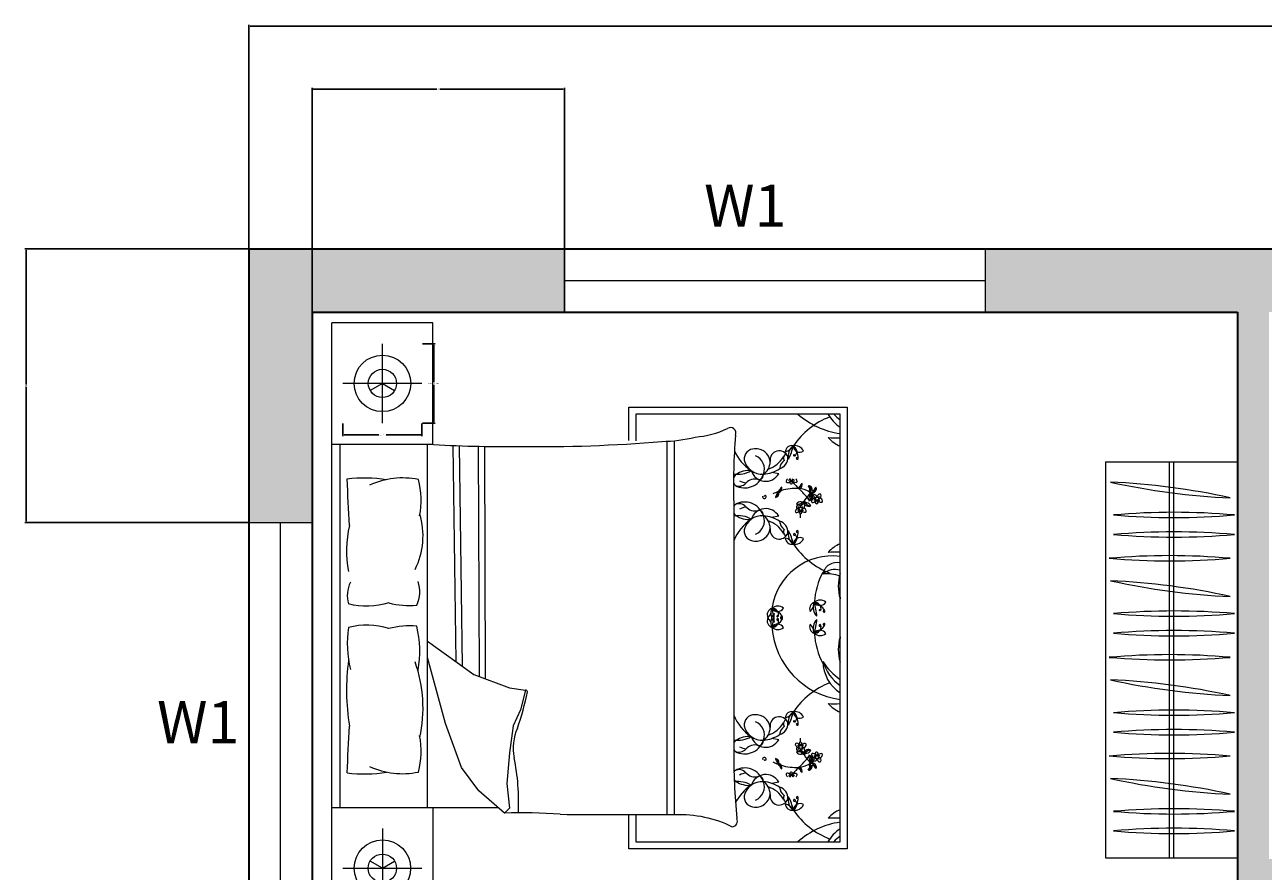
# Model space of a CAD drawing. Units: inches. Extents: x 5 to 421, y -617 to 43.
# Tile 12 of 15: x 5 to 182, y -78 to 43. Entities that reach past the tile are written whole.
import ezdxf

# ---------------------------------------------------------------- set-up
doc = ezdxf.new("R2010")
doc.units = ezdxf.units.IN
doc.header["$MEASUREMENT"] = 0
for name, color, linetype, lineweight in [('A-ANNO-DIMS', 2, 'Continuous', 18), ('A-ANNO-TEXT', 7, 'Continuous', 18), ('A-FLOR-CASE', 8, 'Continuous', 18), ('A-FURN', 8, 'Continuous', 13), ('A-GLAZ', 4, 'Continuous', 18), ('A-WALL', 7, 'Continuous', 35)]:
    doc.layers.add(name, color=color, linetype=linetype, lineweight=lineweight)
doc.layers.add('A-WALL-PATT', color=251, linetype='Continuous', lineweight=13, true_color=0x636466)
doc.styles.get("Standard").update_dxf_attribs({"font": 'arial.ttf'})
doc.dimstyles.get("Standard").update_dxf_attribs({"dimtxt": 0.18, "dimasz": 0.18, "dimexe": 0.18, "dimexo": 0.0625, "dimgap": 0.09, "dimtad": 0, "dimtih": 1, "dimtoh": 1, "dimdec": 0, "dimzin": 0, "dimdsep": 46, "dimlunit": 3, "dimtxsty": 'Standard', "dimcen": 0.09, "dimadec": 0, "dimazin": 0, "dimtfac": 1, "dimtdec": 0, "dimtofl": 0, "dimtmove": 0, "dimatfit": 3, "dimfxl": 1, "dimtolj": 1, "dimtzin": 0, "dimarcsym": 0})

# ---------------------------------------------------------------- blocks, each defined once
blk = doc.blocks.new('WINDOW-W1-60')
for p, q in [((0, 9), (60, 9)), ((0, 0), (0, 9)), ((60, 9), (60, 0)), ((0, 4.5), (60, 4.5)), ((60, 0), (0, 0))]:
    blk.add_line(p, q)
blk = doc.blocks.new('WARDROBE-56')
for p, q in [((0, 56.49), (0, 0)), ((0, 56.49), (18.83, 56.49)), ((9.1, 56.49), (9.1, 0)), ((9.73, 56.49), (9.73, 0)), ((18.83, 56.49), (18.83, 0)), ((0, 0), (18.83, 0))]:
    blk.add_line(p, q)
for centre, start, end in [((22.14, 150.32), 257.508, 267.5023), ((-3.61, -45.4), 77.508, 87.5023), ((9.79, -49.81), 85.0028, 94.9972), ((9.79, 147.6), 265.0028, 274.9972), ((9.79, -52.6), 85.0028, 94.9972), ((9.79, 144.81), 265.0028, 274.9972), ((9.18, -55.99), 85.0028, 94.9972), ((9.18, 141.42), 265.0028, 274.9972), ((22.14, 136.25), 257.508, 267.5023), ((-3.61, -59.47), 77.508, 87.5023), ((9.79, -63.88), 85.0028, 94.9972), ((9.79, 133.52), 265.0028, 274.9972), ((9.79, -66.67), 85.0028, 94.9972), ((9.79, 130.73), 265.0028, 274.9972), ((9.18, -70.11), 85.0028, 94.9972), ((9.18, 127.29), 265.0028, 274.9972), ((-3.61, -73.6), 77.508, 87.5023), ((22.14, 122.12), 257.508, 267.5023), ((9.79, -78.01), 85.0028, 94.9972), ((9.79, 119.4), 265.0028, 274.9972), ((9.79, -80.8), 85.0028, 94.9972), ((9.79, 116.61), 265.0028, 274.9972), ((9.18, -84.19), 85.0028, 94.9972), ((9.18, 113.22), 265.0028, 274.9972), ((-3.61, -87.67), 77.508, 87.5023), ((22.14, 108.05), 257.508, 267.5023), ((9.79, -92.08), 85.0028, 94.9972), ((9.79, 105.32), 265.0028, 274.9972), ((9.79, -94.87), 85.0028, 94.9972), ((9.79, 102.53), 265.0028, 274.9972)]:
    blk.add_arc(centre, 99.08, start, end)
blk = doc.blocks.new('BEDSIDE-LAMP-DOUBLE')
for p, q in [((5.65, 0), (5.65, 11.29)), ((11.29, 5.65), (0, 5.65))]:
    blk.add_line(p, q)
for points in [[(5.65, 5.65), (3.9, 4.64)], [(5.65, 5.65), (7.39, 4.64)]]:
    blk.add_lwpolyline(points)
for radius in [4.03, 2.02]:
    blk.add_circle((5.65, 5.65), radius)
blk = doc.blocks.new('*D48')
at = {"layer": 'A-ANNO-DIMS', "color": 0, "lineweight": -2, "transparency": 16777216}
for p, q in [((62.17, -2.65), (63.98, -2.65)), ((63.8, -2.83), (63.8, -8.11)), ((63.8, -13.76), (63.8, -8.48)), ((62.17, -13.94), (63.98, -13.94))]:
    blk.add_line(p, q, dxfattribs=at)
at = {"layer": 'A-ANNO-DIMS', "color": 0, "transparency": 16777216}
for points in [[(63.77, -2.83), (63.83, -2.83), (63.8, -2.65)], [(63.77, -13.76), (63.83, -13.76), (63.8, -13.94)]]:
    blk.add_solid(points, dxfattribs=at)
at = {"layer": 'Defpoints', "color": 0, "transparency": 16777216}
for p in [(62.1, -2.65), (63.8, -2.65), (62.1, -13.94)]:
    blk.add_point(p, dxfattribs=at)
at = {"layer": 'A-ANNO-DIMS', "color": 0, "transparency": 16777216, "insert": (63.8, -8.3), "char_height": 0.18, "attachment_point": 5}
blk.add_mtext('\\A1;LAMP 11 TYP.', dxfattribs=at)
blk = doc.blocks.new('*D49')
at = {"layer": 'A-ANNO-DIMS', "color": 0, "lineweight": -2, "transparency": 16777216}
for p, q in [((50.81, -14), (50.81, -15.82)), ((62.1, -14), (62.1, -15.82)), ((50.99, -15.64), (55.94, -15.64)), ((61.92, -15.64), (56.98, -15.64))]:
    blk.add_line(p, q, dxfattribs=at)
at = {"layer": 'A-ANNO-DIMS', "color": 0, "transparency": 16777216}
for points in [[(50.99, -15.61), (50.99, -15.67), (50.81, -15.64)], [(61.92, -15.61), (61.92, -15.67), (62.1, -15.64)]]:
    blk.add_solid(points, dxfattribs=at)
at = {"layer": 'Defpoints', "color": 0, "transparency": 16777216}
for p in [(50.81, -13.94), (62.1, -13.94), (62.1, -15.64)]:
    blk.add_point(p, dxfattribs=at)
at = {"layer": 'A-ANNO-DIMS', "color": 0, "transparency": 16777216, "insert": (56.46, -15.64), "char_height": 0.18, "attachment_point": 5}
blk.add_mtext('\\A1;11 TYP.', dxfattribs=at)
blk = doc.blocks.new('*D54')
at = {"layer": 'A-ANNO-DIMS', "color": 0, "lineweight": -2, "transparency": 16777216}
for p, q in [((37.42, 10.94), (37.42, 42.86)), ((37.6, 42.68), (212.65, 42.68)), ((388.24, 42.68), (213.19, 42.68)), ((388.42, -118.06), (388.42, 42.86))]:
    blk.add_line(p, q, dxfattribs=at)
at = {"layer": 'A-ANNO-DIMS', "color": 0, "transparency": 16777216}
for points in [[(37.6, 42.71), (37.6, 42.65), (37.42, 42.68)], [(388.24, 42.71), (388.24, 42.65), (388.42, 42.68)]]:
    blk.add_solid(points, dxfattribs=at)
at = {"layer": 'Defpoints', "color": 0, "transparency": 16777216}
for p in [(37.42, 42.68), (37.42, 10.88), (388.42, -118.12)]:
    blk.add_point(p, dxfattribs=at)
at = {"layer": 'A-ANNO-DIMS', "color": 0, "transparency": 16777216, "insert": (212.92, 42.68), "char_height": 0.18, "attachment_point": 5}
blk.add_mtext('\\A1;351', dxfattribs=at)
blk = doc.blocks.new('*D55')
at = {"layer": 'A-ANNO-DIMS', "color": 0, "lineweight": -2, "transparency": 16777216}
for p, q in [((370.48, 10.88), (420.4, 10.88)), ((420.22, 10.7), (420.22, -286.69)), ((420.22, -584.44), (420.22, -287.05)), ((169.48, -584.62), (420.4, -584.62))]:
    blk.add_line(p, q, dxfattribs=at)
at = {"layer": 'A-ANNO-DIMS', "color": 0, "transparency": 16777216}
for points in [[(420.19, 10.7), (420.25, 10.7), (420.22, 10.88)], [(420.19, -584.44), (420.25, -584.44), (420.22, -584.62)]]:
    blk.add_solid(points, dxfattribs=at)
at = {"layer": 'Defpoints', "color": 0, "transparency": 16777216}
for p in [(370.42, 10.88), (169.42, -584.62), (420.22, -584.62)]:
    blk.add_point(p, dxfattribs=at)
at = {"layer": 'A-ANNO-DIMS', "color": 0, "transparency": 16777216, "insert": (420.22, -286.87), "char_height": 0.18, "attachment_point": 5}
blk.add_mtext('\\A1;595.5', dxfattribs=at)
blk = doc.blocks.new('*D56')
at = {"layer": 'A-ANNO-DIMS', "color": 0, "lineweight": -2, "transparency": 16777216}
for p, q in [((46.42, 1.94), (46.42, 33.86)), ((46.6, 33.68), (64.2, 33.68)), ((82.24, 33.68), (64.64, 33.68)), ((82.42, 1.94), (82.42, 33.86))]:
    blk.add_line(p, q, dxfattribs=at)
at = {"layer": 'A-ANNO-DIMS', "color": 0, "transparency": 16777216}
for points in [[(46.6, 33.71), (46.6, 33.65), (46.42, 33.68)], [(82.24, 33.71), (82.24, 33.65), (82.42, 33.68)]]:
    blk.add_solid(points, dxfattribs=at)
at = {"layer": 'Defpoints', "color": 0, "transparency": 16777216}
for p in [(82.42, 33.68), (46.42, 1.88), (82.42, 1.88)]:
    blk.add_point(p, dxfattribs=at)
at = {"layer": 'A-ANNO-DIMS', "color": 0, "transparency": 16777216, "insert": (64.42, 33.68), "char_height": 0.18, "attachment_point": 5}
blk.add_mtext('\\A1;36', dxfattribs=at)
blk = doc.blocks.new('*D60')
at = {"layer": 'A-ANNO-DIMS', "color": 0, "lineweight": -2, "transparency": 16777216}
for p, q in [((37.36, 10.88), (5.44, 10.88)), ((5.62, 10.7), (5.62, -8.44)), ((5.62, -27.94), (5.62, -8.8)), ((37.36, -28.12), (5.44, -28.12))]:
    blk.add_line(p, q, dxfattribs=at)
at = {"layer": 'A-ANNO-DIMS', "color": 0, "transparency": 16777216}
for points in [[(5.59, 10.7), (5.65, 10.7), (5.62, 10.88)], [(5.59, -27.94), (5.65, -27.94), (5.62, -28.12)]]:
    blk.add_solid(points, dxfattribs=at)
at = {"layer": 'Defpoints', "color": 0, "transparency": 16777216}
for p in [(37.42, 10.88), (5.62, -28.12), (37.42, -28.12)]:
    blk.add_point(p, dxfattribs=at)
at = {"layer": 'A-ANNO-DIMS', "color": 0, "transparency": 16777216, "insert": (5.62, -8.62), "char_height": 0.18, "attachment_point": 5}
blk.add_mtext('\\A1;39', dxfattribs=at)

msp = doc.modelspace()

# ---------------------------------------------------------------- hatches: boundary and pattern name
at = {"layer": 'A-WALL-PATT'}
h = msp.add_hatch(color=256, dxfattribs=at)
h.dxf.hatch_style = 1
h.paths.add_polyline_path([(46.4196, -88.1188), (37.4196, -88.1188), (37.4196, -166.6119), (46.4196, -166.6119), (46.4196, -122.6188), (135.4196, -122.6188), (135.4196, -120.3688), (135.4196, -118.1188), (46.4196, -118.1188)])
h.paths.add_polyline_path([(82.4196, 10.8812), (37.4196, 10.8812), (37.4196, -28.1188), (46.4196, -28.1188), (46.4196, 1.8812), (82.4196, 1.8812)])
h.paths.add_polyline_path([(215.5968, 10.8812), (142.4196, 10.8812), (142.4196, 1.8812), (178.4196, 1.8812), (178.4196, -118.1188), (175.4196, -118.1188), (175.4196, -122.6188), (182.9196, -122.6188), (182.9196, -80.6188), (211.9196, -80.6188), (211.9196, -78.3688), (211.9196, -76.1188), (182.9196, -76.1188), (182.9196, 1.8812), (215.5968, 1.8812)])
h.paths.add_polyline_path([(274.4196, 10.8812), (239.5968, 10.8812), (239.5968, 1.8812), (242.9196, 1.8812), (242.9196, -76.1188), (239.9196, -76.1188), (239.9196, -80.6188), (242.9196, -80.6188), (242.9196, -83.6188), (247.4196, -83.6188), (247.4196, 1.8812), (274.4196, 1.8812)])
h.paths.add_polyline_path([(370.4196, 10.8812), (334.4196, 10.8812), (334.4196, 1.8812), (361.4196, 1.8812), (361.4196, -28.1188), (370.4196, -28.1188)])
h.paths.add_polyline_path([(370.4196, -88.1188), (361.4196, -88.1188), (361.4196, -118.1188), (247.4196, -118.1188), (247.4196, -115.1188), (242.9196, -115.1188), (242.9196, -118.1188), (220.4196, -118.1188), (220.4196, -158.6188), (224.9196, -158.6188), (224.9196, -122.6188), (326.9196, -122.6188), (326.9196, -170.7662), (331.4196, -170.7662), (331.4196, -122.6188), (370.4196, -122.6188)])
h.paths.add_polyline_path([(388.4196, -122.6188), (388.4196, -118.1188), (379.4196, -118.1188), (379.4196, -122.6188), (379.4196, -154.8688), (388.4196, -154.8688)])
h.paths.add_polyline_path([(388.4196, -214.8688), (379.4196, -214.8688), (379.4196, -247.1188), (388.4196, -247.1188)])
h.paths.add_polyline_path([(371.0265, -242.6188), (331.4196, -242.6188), (331.4196, -239.6188), (326.9196, -239.6188), (326.9196, -242.6188), (224.9196, -242.6188), (224.9196, -206.6188), (220.4196, -206.6188), (220.4196, -343.6188), (224.9196, -343.6188), (229.4196, -343.6188), (229.4196, -247.1188), (261.5265, -247.1188), (261.5265, -276.1188), (263.7765, -276.1188), (266.0265, -276.1188), (266.0265, -247.1188), (362.0265, -247.1188), (362.0265, -265.1188), (371.0265, -265.1188), (371.0265, -247.1188)])
h.paths.add_polyline_path([(371.0265, -289.1188), (362.0265, -289.1188), (362.0265, -307.1188), (266.0265, -307.1188), (266.0265, -304.1188), (261.5265, -304.1188), (261.5265, -307.1188), (261.5265, -311.6188), (362.0265, -311.6188), (362.0265, -353.6188), (371.0265, -353.6188)])
h.paths.add_polyline_path([(371.0265, -413.6188), (362.0265, -413.6188), (362.0265, -455.6188), (325.7231, -455.6188), (325.7231, -464.6188), (361.4196, -464.6188), (371.0265, -464.6188)])
h.paths.add_polyline_path([(265.7231, -455.6188), (229.4196, -455.6188), (229.4196, -383.6188), (220.4196, -383.6188), (220.4196, -386.6188), (207.4649, -386.6188), (207.4649, -395.6188), (220.4196, -395.6188), (220.4196, -455.6188), (216.0568, -455.6188), (216.0568, -464.6188), (265.7231, -464.6188)])
h.paths.add_polyline_path([(169.4196, -386.6188), (137.9196, -386.6188), (137.9196, -395.6188), (160.4196, -395.6188), (160.4196, -424.2032), (169.4196, -424.2032)])
h.paths.add_polyline_path([(169.4196, -453.7423), (160.4196, -453.7423), (160.4196, -464.6188), (169.4196, -464.6188)])
h.paths.add_polyline_path([(46.4196, -575.6188), (37.4196, -575.6188), (37.4196, -584.6188), (46.4196, -584.6188)])
h.paths.add_polyline_path([(169.4196, -575.6188), (160.4196, -575.6188), (160.4196, -579.5504), (160.4196, -584.6188), (169.4196, -584.6188)])
h.paths.add_polyline_path([(46.4196, -226.6119), (37.4196, -226.6119), (37.4196, -292.8008), (46.4196, -292.8008)])
h.paths.add_polyline_path([(46.4196, -352.8008), (37.4196, -352.8008), (37.4196, -395.6188), (77.9196, -395.6188), (77.9196, -386.6188), (46.4196, -386.6188)])

# ---------------------------------------------------------------- linework, layer by layer
at = {"layer": 'A-FURN'}
for p, q in [((49.2533, -86.083), (49.2533, 0.3477)), ((91.622, -16.4566), (91.622, -11.6634)), ((91.622, -11.6634), (122.7569, -11.6634)), ((122.7569, -11.6634), (122.7569, -74.675)), ((92.6236, -12.665), (92.6236, -16.4748)), ((121.7553, -12.665), (92.6236, -12.665)), ((121.7553, -73.6735), (121.7553, -12.665)), ((50.3628, -16.9384), (50.3628, -68.7969)), ((62.9119, -68.7969), (62.9119, -16.9384)), ((66.5026, -17.1704), (66.9339, -47.9422)), ((67.3896, -17.204), (67.8327, -48.5879)), ((70.1108, -17.2486), (70.2412, -50.0686)), ((70.9982, -17.2442), (71.1342, -50.4075)), ((97.0125, -16.5457), (97.0125, -69.7927)), ((98.0906, -16.4637), (98.0906, -69.7929)), ((112.9927, -21.1822), (112.016, -20.9911)), ((106.5805, -25.3215), (106.5805, -60.4138)), ((112.9927, -27.2228), (112.016, -27.4139)), ((62.9119, -45.0527), (69.5046, -49.789)), ((65.4807, -56.7913), (62.9119, -47.3665)), ((69.5046, -49.789), (74.5781, -51.7146)), ((74.5781, -51.7146), (76.8525, -52.0647)), ((76.8525, -52.0647), (76.1527, -54.8657)), ((76.1527, -54.8657), (75.103, -57.1415)), ((67.7551, -63.0935), (65.4807, -56.7913)), ((75.103, -57.1415), (74.5781, -60.9928)), ((112.9927, -59.1157), (112.016, -58.9246)), ((74.5781, -60.9928), (74.2283, -65.3693)), ((70.2044, -66.4196), (67.7551, -63.0935)), ((112.9927, -65.1562), (112.016, -65.3473)), ((73.8783, -69.5707), (70.2044, -66.4196)), ((74.2283, -65.3693), (74.5781, -68.8704)), ((49.2533, -68.7969), (72.9761, -68.7969)), ((74.5781, -68.8704), (73.8783, -69.5707)), ((91.622, -74.675), (91.622, -69.7861)), ((92.6236, -69.788), (92.6236, -73.6735)), ((92.6236, -73.6735), (121.7553, -73.6735)), ((122.7569, -74.675), (91.622, -74.675))]:
    msp.add_line(p, q, dxfattribs=at)
for points in [[(49.2533, -16.9384), (63.6585, -16.9384), (63.6585, 0.3477), (49.2533, 0.3477)], [(63.6585, -68.7969), (63.6585, -86.083), (49.2533, -86.083)]]:
    msp.add_lwpolyline(points, dxfattribs=at)
for points in [[(96.3321, -16.5695, 0.05611182), (101.0874, -15.9424, 0.09534134), (105.6678, -14.7276)], [(51.4075, -21.9027, -0.07489676), (57.0529, -22.0076, 0.47281659)], [(57.3687, -39.5817, -0.14098958), (51.6093, -39.7546, -0.23524475)], [(57.3687, -43.2726, 0.14098958), (51.6093, -43.0997, 0.23524475)], [(51.4075, -63.8326, 0.07489676), (57.0529, -63.7277, -0.47281659)], [(81.7924, -69.7515, 0.00124232), (98.1917, -69.7929, -0.12720156), (106.3647, -71.5256)]]:
    msp.add_lwpolyline(points, format="xyb", dxfattribs=at)
for centre in [(118.4447, -24.7359), (116.1246, -26.1756), (116.1246, -60.1628), (118.4447, -61.6026)]:
    msp.add_circle(centre, 0.2201, dxfattribs=at)
for centre, radius, start, end in [((124.3922, -23.5719), 11.2866, 111.409207, 145.613455), ((123.2763, -4.2623), 11.2866, 228.114397, 262.255043), ((124.7877, -9.9244), 5.4997, 209.888429, 236.538275), ((125.8131, -7.9456), 6.8536, 223.518578, 233.696435), ((106.1063, -15.382), 0.7878, 336.521858, 123.826416), ((190.6427, -22.6746), 84.1038, 175.240242, 181.803508), ((73.4749, 138.0038), 155.3018, 266.099968, 270.928176), ((79.1213, 185.2819), 202.5838, 269.114536, 274.873507), ((109.5261, -19.0821), 1.4593, 88.94622, 185.514429), ((109.7349, -19.6805), 2.0654, 7.114253, 95.055148), ((114.8559, -18.1065), 0.9357, 76.272036, 177.048413), ((113.4322, -16.1937), 1.9278, 284.703123, 328.617328), ((116.1209, -18.6454), 1.7844, 125.765707, 194.534651), ((107.3699, -15.4863), 7.8958, 332.81761, 347.482743), ((115.3444, -18.4205), 1.2516, 20.961322, 102.288469), ((116.0202, -17.1694), 0.9426, 181.713105, 301.536686), ((112.929, -19.0762), 2.8544, 2.064805, 41.159835), ((114.6491, -18.0152), 0.9233, 316.223807, 62.317301), ((123.5155, -13.0046), 4.589, 221.04544, 247.445257), ((121.0491, -0.434), 15.6157, 266.348095, 272.591893), ((112.6671, -15.2714), 6.5415, 203.645326, 236.332878), ((110.6057, -18.6341), 2.5996, 193.079005, 274.706656), ((108.9518, -20.4923), 2.0058, 338.577852, 68.418133), ((109.2759, -19.3213), 2.5107, 305.959859, 357.640897), ((110.2076, -16.6335), 4.0805, 288.295495, 328.738626), ((113.0629, -19.2053), 1.2971, 19.131157, 189.736024), ((112.6725, -18.8941), 1.6198, 285.695503, 4.030982), ((114.8259, -20.6388), 1.7252, 128.417454, 173.833797), ((114.4684, -18.9383), 0.795, 126.731946, 206.024452), ((115.1809, -18.556), 0.0736, 20.266709, 316.227077), ((115.6414, -18.9784), 0.1402, 168.516605, 2.064805), ((115.5708, -18.9641), 0.0681, 52.059106, 168.516605), ((107.22, -17.6706), 3.5809, 259.248989, 301.178216), ((108.7748, -24.0384), 3.3333, 85.269627, 124.214953), ((111.1301, -20.1108), 2.1487, 196.866299, 330.091459), ((110.5365, -16.5953), 4.6382, 273.492404, 303.711716), ((-771.1281, -69.5429), 823.914, 2.8502247, 3.3147907), ((59.3194, -32.9142), 11.1396, 78.241659, 114.8684), ((50.3959, -24.9859), 11.5828, 348.963113, 14.896067), ((107.5367, -22.1059), 1.0409, 196.634335, 225.548308), ((107.5367, -22.1059), 1.0409, 127.675028, 162.581425), ((108.1504, -20.444), 2.7543, 240.8249, 340.717823), ((107.3303, -21.6659), 1.2933, 246.164593, 318.434694), ((108.6488, -20.0282), 2.4845, 240.085135, 262.564012), ((109.6237, -23.6996), 1.7719, 74.852873, 138.434694), ((110.2269, -21.4714), 0.5364, 254.852873, 12.695942), ((108.7748, -24.0384), 3.3333, 53.65552, 57.29887), ((114.2136, -22.2785), 0.1701, 125.075197, 284.764439), ((114.4756, -22.2129), 0.3671, 127.364203, 168.436272), ((114.1879, -21.9181), 0.5293, 277.496845, 341.273729), ((114.6082, -22.1651), 0.2102, 88.132531, 178.891946), ((115.0311, -22.3883), 0.455, 136.346175, 189.651304), ((114.7695, -22.4328), 0.1897, 189.651304, 312.320848), ((114.8165, -21.9085), 0.2201, 183.276835, 356.723165), ((115.504, -22.302), 0.7206, 164.282907, 186.914838), ((114.6547, -22.3068), 0.3602, 312.320848, 40.211082), ((115.4174, -21.9008), 0.5115, 201.638236, 274.946963), ((114.74, -22.6007), 0.6683, 42.389629, 66.572429), ((121.4818, -17.3122), 8.2064, 217.954095, 226.845875), ((115.2241, -22.2084), 0.3634, 10.959737, 52.237914), ((115.4469, -22.2422), 0.1689, 274.946963, 37.526288), ((115.8999, -22.8852), 0.4148, 265.713146, 351.656778), ((114.9877, -22.0331), 1.3887, 313.692881, 321.789879), ((116.5238, -22.9811), 0.4538, 115.53786, 168.674386), ((114.9839, -22.3284), 1.3661, 329.344007, 349.741218), ((113.8917, -22.6429), 2.4375, 352.869762, 1.673614), ((117.3198, -23.1343), 0.2458, 33.097874, 123.136405), ((111.9059, -26.5995), 6.4304, 31.115593, 34.811802), ((116.9636, -23.5558), 0.6654, 2.31716, 70.520132), ((110.9381, -24.4317), 0.2709, 169.586441, 349.561551), ((111.0406, -24.4506), 0.1666, 349.561551, 167.29493), ((115.391, -30.4415), 7.1586, 110.105922, 116.996805), ((112.9899, -24.5411), 0.4538, 129.505588, 182.642118), ((111.6873, -23.492), 1.3661, 308.438755, 328.835967), ((111.4487, -22.3808), 2.4375, 296.506361, 305.310211), ((111.4288, -23.6348), 1.3887, 336.390094, 344.487092), ((112.9421, -23.9889), 0.1761, 83.945725, 185.621623), ((112.2364, -23.8241), 0.7244, 328.835967, 0.814121), ((112.6107, -24.0365), 0.4148, 306.523195, 32.466832), ((113.1063, -23.7147), 0.1761, 112.558349, 214.234253), ((112.9917, -23.4002), 0.4148, 265.713146, 351.656778), ((112.6277, -23.1705), 0.7244, 297.365857, 329.344007), ((112.0794, -22.548), 1.3887, 313.692881, 321.789879), ((113.6156, -23.4961), 0.4538, 115.53786, 168.674386), ((112.0757, -22.8433), 1.3661, 329.344007, 349.741218), ((115.391, -30.4415), 7.1586, 86.172317, 106.415821), ((110.9835, -23.1578), 2.4375, 352.869762, 1.673614), ((116.0145, -23.1998), 0.1761, 112.558349, 214.234253), ((115.536, -22.6556), 0.7244, 297.365857, 329.344007), ((115.5714, -26.8752), 3.5887, 60.795916, 85.243979), ((107.9299, -32.0417), 11.8096, 37.825561, 47.758756), ((120.338, -27.2444), 4.3048, 130.182023, 149.455983), ((117.9678, -24.7927), 0.7098, 139.381187, 199.995928), ((116.6434, -24.2774), 1.0033, 310.936473, 22.769517), ((117.1042, -24.3334), 0.729, 285.64837, 332.295742), ((117.513, -23.7196), 0.192, 135.735421, 318.129663), ((117.1933, -23.408), 0.2545, 315.735421, 31.115593), ((116.9808, -23.9462), 0.5905, 319.381187, 5.545644), ((117.6571, -23.7187), 0.192, 68.245218, 250.639457), ((117.2151, -23.4817), 0.573, 352.600826, 57.184524), ((119.2622, -27.3284), 3.8337, 111.708712, 116.218055), ((115.5714, -26.8752), 3.5887, 47.508292, 55.996664), ((117.7628, -23.3525), 0.573, 252.804199, 349.694321), ((117.2153, -24.3783), 0.6099, 331.183768, 51.679176), ((117.8225, -23.3041), 0.2545, 248.245218, 323.62539), ((118.1038, -25.0402), 0.3671, 93.634966, 168.436272), ((118.057, -24.4595), 0.2157, 138.29465, 276.247442), ((117.5981, -23.1484), 0.6654, 291.708712, 3.029927), ((118.1385, -24.4929), 0.3002, 358.571889, 143.895444), ((112.8499, -19.6413), 6.4304, 323.62539, 327.321597), ((118.3133, -24.2566), 0.303, 208.849254, 269.935492), ((118.0551, -24.3286), 0.3462, 274.212295, 318.15875), ((118.1238, -23.3161), 0.2458, 325.607669, 55.646202), ((119.1097, -24.6771), 0.694, 121.950101, 165.244186), ((118.6303, -24.4099), 0.1458, 262.868017, 7.093987), ((118.6127, -24.2877), 0.4344, 278.561414, 22.591427), ((118.8523, -25.0357), 0.3634, 10.959737, 118.780415), ((118.8579, -24.2733), 0.2181, 44.373191, 121.950101), ((107.5367, -26.2991), 1.0409, 134.451692, 156.714357), ((108.1504, -27.961), 2.7543, 19.282177, 119.1751), ((107.3303, -26.7391), 1.2933, 41.565306, 113.835407), ((108.6488, -28.3768), 2.4845, 97.435988, 119.914865), ((109.6237, -24.7054), 1.7719, 221.565306, 285.147127), ((111.1301, -28.2942), 2.1487, 29.908541, 163.133701), ((110.2269, -26.9336), 0.5364, 347.304058, 105.147127), ((115.5217, -26.5456), 0.1701, 125.075197, 284.764439), ((115.7837, -26.48), 0.3671, 93.634966, 168.436272), ((115.7975, -24.4906), 1.0033, 253.630094, 325.463139), ((116.0792, -25.8834), 0.7098, 82.074807, 142.689549), ((115.9993, -24.9086), 0.729, 228.34199, 274.989364), ((115.7369, -25.8992), 0.2157, 138.29465, 276.247442), ((115.496, -26.1852), 0.5293, 277.496845, 341.273729), ((115.8184, -25.9326), 0.3002, 358.571889, 143.895444), ((115.9163, -26.4321), 0.2102, 88.132531, 178.891946), ((115.9932, -25.6963), 0.303, 208.849254, 269.935492), ((115.735, -25.7683), 0.3462, 274.212295, 318.15875), ((116.3392, -26.6554), 0.455, 136.346175, 189.651304), ((116.0214, -25.0264), 0.6099, 273.877392, 357.150123), ((116.8121, -26.569), 0.7206, 164.282907, 186.914838), ((116.7896, -26.1168), 0.694, 121.950101, 165.244186), ((116.2585, -24.5956), 0.5905, 262.074807, 308.239267), ((115.9628, -26.5738), 0.3602, 312.320848, 40.211082), ((116.7255, -26.1679), 0.5115, 201.638236, 274.946963), ((116.3102, -25.8496), 0.1458, 262.868017, 7.093987), ((116.0481, -26.8678), 0.6683, 42.389629, 66.572429), ((116.2926, -25.7274), 0.4344, 278.561414, 22.591427), ((116.5322, -26.4755), 0.3634, 10.959737, 118.780415), ((120.338, -27.2444), 4.3048, 156.152261, 156.949926), ((116.5377, -25.713), 0.2181, 44.373191, 121.950101), ((117.2108, -25.2004), 0.6099, 181.4625, 249.4747), ((117.107, -24.7198), 0.5905, 215.112828, 261.277285), ((117.5788, -24.7512), 1.0033, 197.888952, 269.721997), ((116.755, -26.5092), 0.1689, 274.946963, 37.526288), ((117.2657, -25.0939), 0.729, 248.362726, 295.010099), ((116.9098, -26.005), 0.7098, 20.662543, 81.277285), ((117.8418, -25.1058), 0.1701, 125.075197, 284.764439), ((117.8161, -24.7455), 0.5293, 277.496845, 341.273729), ((118.2364, -24.9924), 0.2102, 88.132531, 178.891946), ((118.6593, -25.2157), 0.455, 136.346175, 189.651304), ((118.3977, -25.2602), 0.1897, 189.651304, 312.320848), ((119.1322, -25.1293), 0.7206, 164.282907, 186.914838), ((118.2829, -25.1341), 0.3602, 312.320848, 40.211082), ((119.0456, -24.7281), 0.5115, 201.638236, 274.946963), ((118.3682, -25.428), 0.6683, 42.389629, 66.572429), ((119.0751, -25.0695), 0.1689, 274.946963, 37.526288), ((51.2494, -29.9849), 11.0022, 333.876108, 16.174639), ((107.5367, -26.2991), 1.0409, 203.285643, 232.324972), ((107.22, -30.7344), 3.5809, 58.821784, 100.286655), ((112.6671, -33.1336), 6.5415, 123.667122, 158.505868), ((108.7748, -24.3666), 3.3333, 235.785047, 274.730373), ((110.6057, -29.7709), 2.5996, 85.293344, 166.920995), ((108.9518, -27.9127), 2.0058, 291.581867, 21.422148), ((108.7748, -24.3666), 3.3333, 302.70113, 306.34448), ((109.2759, -29.0837), 2.5107, 2.359103, 54.040141), ((110.5365, -31.8097), 4.6382, 56.288284, 86.507596), ((110.2076, -31.7715), 4.0805, 31.261374, 71.704505), ((114.8259, -27.7662), 1.7252, 186.166203, 231.582546), ((112.6725, -29.5109), 1.6198, 355.969018, 74.304497), ((116.0776, -26.6999), 0.1897, 189.651304, 312.320848), ((120.338, -27.2444), 4.3048, 175.241474, 182.892907), ((66.531, -32.161), 15.1939, 166.342714, 191.1841), ((109.5261, -29.3229), 1.4593, 174.485571, 271.05378), ((109.7349, -28.7245), 2.0654, 264.944852, 352.885747), ((113.0629, -29.1997), 1.2971, 170.263976, 340.868843), ((114.4684, -29.4667), 0.795, 153.975548, 233.268054), ((116.1209, -29.7596), 1.7844, 165.465349, 234.234293), ((107.3699, -32.9187), 7.8958, 12.517257, 27.18239), ((112.929, -29.3288), 2.8544, 318.840165, 357.935195), ((114.6491, -30.3898), 0.9233, 297.682699, 43.776193), ((115.2276, -29.8355), 0.1221, 43.776193, 339.718346), ((115.6414, -29.4266), 0.1402, 357.935195, 191.483395), ((115.5708, -29.4409), 0.0681, 191.483395, 307.940894), ((114.8559, -30.2985), 0.9357, 182.951587, 283.727964), ((113.4322, -32.2113), 1.9278, 31.382672, 75.296877), ((116.0202, -31.2356), 0.9426, 58.463314, 178.286895), ((115.3444, -29.9845), 1.2516, 257.711531, 339.038678), ((124.3922, -24.8331), 11.2866, 214.386545, 248.590793), ((123.5155, -35.4004), 4.589, 112.554743, 138.95456), ((120.6701, -41.6265), 8.7351, 82.863554, 171.819659), ((121.0491, -47.971), 15.6157, 87.408107, 93.651905), ((129.3216, -40.3975), 11.2866, 152.585402, 175.537671), ((121.2786, -35.8615), 2.0259, 76.389819, 169.073851), ((121.0004, -37.3841), 2.5618, 72.860876, 131.904868), ((55.7172, -38.5687), 4.2757, 153.343742, 196.102557), ((57.2087, -37.9905), 4.5819, 335.01826, 18.540728), ((119.8719, -40.497), 5.0532, 68.117032, 96.619536), ((127.6897, -37.241), 6.2062, 162.979799, 196.456893), ((130.8882, -39.6999), 9.1773, 174.364262, 175.621276), ((60.2574, -29.3932), 10.5901, 254.170723, 275.987112), ((112.2849, -41.2821), 0.9357, 106.196251, 206.972629), ((110.0968, -40.3345), 1.9278, 314.627337, 358.541544), ((113.6501, -41.1181), 1.7844, 155.689918, 224.458869), ((112.8649, -41.3106), 1.2516, 50.885535, 132.212682), ((112.8264, -39.8891), 0.9426, 211.637318, 331.460901), ((112.06, -41.3061), 0.9233, 346.14802, 92.241514), ((111.0986, -43.0838), 2.8544, 31.989022, 71.084052), ((104.4897, -42.7456), 7.8958, 2.741826, 17.406963), ((118.3302, -40.4179), 0.9357, 106.196251, 206.972629), ((116.1421, -39.4703), 1.9278, 314.627337, 358.541544), ((119.6954, -40.254), 1.7844, 155.689918, 224.458869), ((118.9102, -40.4464), 1.2516, 50.885535, 132.212682), ((118.8717, -39.025), 0.9426, 211.637318, 331.460901), ((118.1053, -40.442), 0.9233, 346.14802, 92.241514), ((117.1439, -42.2197), 2.8544, 31.989022, 71.084052), ((110.535, -41.8815), 7.8958, 2.741826, 17.406963), ((118.8361, -40.6454), 0.0736, 50.190924, 346.020882), ((137.1758, -44.5334), 16.4001, 160.097156, 160.278285), ((112.2849, -42.1753), 0.9357, 153.027371, 253.803749), ((110.0968, -43.1229), 1.9278, 1.458456, 45.372663), ((113.6501, -42.3393), 1.7844, 135.541131, 204.310082), ((104.4897, -40.7118), 7.8958, 342.593037, 357.258174), ((111.0986, -40.3736), 2.8544, 288.915948, 328.010978), ((112.06, -42.1513), 0.9233, 267.758486, 13.85198), ((112.8379, -41.9595), 0.1221, 13.85198, 309.924541), ((112.7908, -41.5096), 0.0736, 50.190924, 346.020882), ((113.3322, -41.6687), 0.0681, 81.983321, 198.440821), ((113.3322, -41.7887), 0.0681, 161.559179, 278.016679), ((113.4006, -41.6459), 0.1402, 198.440821, 31.989022), ((113.4006, -41.8115), 0.1402, 328.010978, 161.559179), ((119.6954, -43.2034), 1.7844, 135.541131, 204.310082), ((110.535, -41.576), 7.8958, 342.593037, 357.258174), ((119.3775, -40.8046), 0.0681, 81.983321, 198.440821), ((119.4459, -40.7818), 0.1402, 198.440821, 31.989022), ((66.842, -45.3695), 15.4009, 171.524927, 193.959959), ((60.2574, -53.4611), 10.5901, 84.012888, 105.829277), ((46.5491, -46.5189), 15.2418, 349.861689, 13.623756), ((112.8264, -43.5683), 0.9426, 28.539099, 148.362682), ((112.8649, -42.1468), 1.2516, 227.787318, 309.114465), ((123.2763, -42.1957), 11.2866, 184.462329, 262.255043), ((118.3302, -43.0395), 0.9357, 153.027371, 253.803749), ((116.1421, -43.9871), 1.9278, 1.458456, 45.372663), ((117.1439, -41.2378), 2.8544, 288.915948, 328.010978), ((118.1053, -43.0154), 0.9233, 267.758486, 13.85198), ((118.8717, -44.4325), 0.9426, 28.539099, 148.362682), ((118.9102, -43.011), 1.2516, 227.787318, 309.114465), ((129.3216, -43.0599), 11.2866, 184.462329, 207.414598), ((118.8832, -42.8236), 0.1221, 13.85198, 309.924541), ((119.3775, -42.6528), 0.0681, 161.559179, 278.016679), ((119.4459, -42.6756), 0.1402, 328.010978, 161.559179), ((127.6897, -46.2164), 6.2062, 163.543107, 197.020201), ((130.8882, -43.7575), 9.1773, 184.378724, 185.635738), ((137.1758, -38.924), 16.4001, 199.721715, 199.902844), ((82.6833, -51.9898), 31.3463, 172.219583, 189.496983), ((42.1628, -54.6521), 20.0894, 348.039745, 19.261524), ((124.7877, -47.8578), 5.4997, 181.271967, 236.538275), ((127.74, -42.2773), 10.1947, 214.012338, 234.053042), ((125.8131, -45.8791), 6.8536, 197.850379, 233.696435), ((124.3922, -61.5054), 11.2866, 111.409207, 145.613455), ((44.1914, -46.0639), 33.5187, 340.119422, 349.33829), ((76.923, -52.261), 0.2086, 358.862345, 109.753635), ((121.0491, -38.3675), 15.6157, 266.348095, 272.591893), ((123.5155, -50.9381), 4.589, 221.04544, 247.445257), ((112.6671, -53.2048), 6.5415, 201.494132, 236.332878), ((109.5261, -57.0155), 1.4593, 88.94622, 185.514429), ((109.7349, -57.6139), 2.0654, 7.114253, 95.055148), ((113.0629, -57.1388), 1.2971, 19.131157, 189.736024), ((114.4684, -56.8717), 0.795, 126.731946, 206.024452), ((114.8559, -56.0399), 0.9357, 76.272036, 177.048413), ((113.4322, -54.1271), 1.9278, 284.703123, 328.617328), ((116.1209, -56.5789), 1.7844, 125.765707, 194.534651), ((107.3699, -53.4197), 7.8958, 332.81761, 347.482743), ((115.3444, -56.3539), 1.2516, 20.961322, 102.288469), ((114.6491, -55.9486), 0.9233, 316.223807, 62.317301), ((112.929, -57.0097), 2.8544, 2.064805, 41.159835), ((116.0202, -55.1028), 0.9426, 181.713105, 301.536686), ((115.1809, -56.4895), 0.0736, 20.266709, 316.227077), ((-771.1281, -16.1924), 823.914, 356.6852093, 357.1497753), ((82.1529, -60.2945), 7.0356, 156.261584, 191.339199), ((110.6057, -56.5675), 2.5996, 193.079005, 274.706656), ((108.9518, -58.4257), 2.0058, 338.577852, 68.418133), ((109.2759, -57.2548), 2.5107, 305.959859, 357.640897), ((110.2076, -54.567), 4.0805, 288.295495, 328.738626), ((112.6725, -56.8275), 1.6198, 285.695503, 4.030982), ((114.8259, -58.5722), 1.7252, 128.417454, 173.833797), ((115.6414, -56.9119), 0.1402, 168.516605, 2.064805), ((115.5708, -56.8975), 0.0681, 52.059106, 168.516605), ((50.3959, -60.7494), 11.5828, 345.103933, 11.036887), ((107.22, -55.6041), 3.5809, 259.713345, 301.178216), ((107.5367, -60.0393), 1.0409, 127.675028, 156.714357), ((108.1504, -58.3774), 2.7543, 240.8249, 340.717823), ((108.7748, -61.9718), 3.3333, 85.269627, 124.214953), ((109.6237, -61.633), 1.7719, 74.852873, 138.434694), ((111.1301, -58.0443), 2.1487, 196.866299, 330.091459), ((110.2269, -59.4049), 0.5364, 254.852873, 12.695942), ((108.7748, -61.9718), 3.3333, 53.65552, 57.29887), ((110.5365, -54.5287), 4.6382, 273.492404, 303.711716), ((115.5217, -59.7929), 0.1701, 75.235561, 234.924803), ((115.7837, -59.8585), 0.3671, 191.563728, 266.365034), ((115.496, -60.1532), 0.5293, 18.726271, 82.503155), ((115.9163, -59.9063), 0.2102, 181.108054, 271.867469), ((116.3392, -59.683), 0.455, 170.348696, 223.653825), ((116.0776, -59.6385), 0.1897, 47.679152, 170.348696), ((120.338, -59.0941), 4.3048, 177.107093, 184.758526), ((116.8121, -59.7694), 0.7206, 173.085162, 195.717093), ((115.9628, -59.7646), 0.3602, 319.788918, 47.679152), ((116.7255, -60.1706), 0.5115, 85.053037, 158.361764), ((116.0481, -59.4707), 0.6683, 293.427571, 317.610371), ((116.5322, -59.863), 0.3634, 241.219585, 349.040263), ((116.755, -59.8292), 0.1689, 322.473712, 85.053037), ((43.2712, -68.0915), 32.6201, 357.45188, 11.339199), ((196.55, -61.4451), 89.9754, 179.343254, 185.688691), ((107.5367, -60.0393), 1.0409, 203.229008, 225.548308), ((107.3303, -59.5994), 1.2933, 246.164593, 318.434694), ((108.6488, -57.9616), 2.4845, 240.085135, 262.564012), ((110.9381, -61.9068), 0.2709, 10.438449, 190.413559), ((112.9899, -61.7973), 0.4538, 177.357882, 230.494412), ((111.6873, -62.8464), 1.3661, 31.164033, 51.561245), ((111.4487, -63.9577), 2.4375, 54.689789, 63.493639), ((115.9993, -61.4299), 0.729, 85.010636, 131.65801), ((115.7975, -61.8479), 1.0033, 34.536861, 106.369906), ((116.0792, -60.455), 0.7098, 217.310451, 277.925193), ((115.7369, -60.4392), 0.2157, 83.752558, 221.70535), ((115.8184, -60.4058), 0.3002, 216.104556, 1.428111), ((115.9932, -60.6422), 0.303, 90.064508, 151.150746), ((115.735, -60.5701), 0.3462, 41.84125, 85.787705), ((107.9299, -54.2967), 11.8096, 312.241244, 322.174439), ((116.0214, -61.3121), 0.6099, 2.849877, 86.122608), ((116.7896, -60.2216), 0.694, 194.755814, 238.049899), ((116.2585, -61.7428), 0.5905, 51.760733, 97.925193), ((116.3102, -60.4888), 0.1458, 352.906013, 97.131983), ((116.2926, -60.611), 0.4344, 337.408573, 81.438586), ((120.338, -59.0941), 4.3048, 203.050074, 203.847739), ((116.5377, -60.6254), 0.2181, 238.049899, 315.626809), ((117.2108, -61.1381), 0.6099, 110.5253, 178.5375), ((117.5788, -61.5872), 1.0033, 90.278003, 162.111048), ((117.107, -61.6187), 0.5905, 98.722715, 144.887172), ((120.338, -59.0941), 4.3048, 210.544017, 229.817977), ((117.2657, -61.2446), 0.729, 64.989901, 111.637274), ((116.9098, -60.3335), 0.7098, 278.722715, 339.337457), ((117.9678, -61.5458), 0.7098, 160.004072, 220.618813), ((116.6434, -62.061), 1.0033, 337.230483, 49.063527), ((117.1042, -62.0051), 0.729, 27.704258, 74.35163), ((117.2153, -61.9601), 0.6099, 308.320824, 28.816232), ((117.8418, -61.2326), 0.1701, 75.235561, 234.924803), ((118.1038, -61.2982), 0.3671, 191.563728, 266.365034), ((118.057, -61.879), 0.2157, 83.752558, 221.70535), ((117.8161, -61.5929), 0.5293, 18.726271, 82.503155), ((118.2364, -61.346), 0.2102, 181.108054, 271.867469), ((118.3133, -62.0819), 0.303, 90.064508, 151.150746), ((118.0551, -62.0098), 0.3462, 41.84125, 85.787705), ((118.6593, -61.1227), 0.455, 170.348696, 223.653825), ((118.3977, -61.0783), 0.1897, 47.679152, 170.348696), ((119.1322, -61.2091), 0.7206, 173.085162, 195.717093), ((118.2829, -61.2043), 0.3602, 319.788918, 47.679152), ((119.0456, -61.6103), 0.5115, 85.053037, 158.361764), ((118.6303, -61.9285), 0.1458, 352.906013, 97.131983), ((118.3682, -60.9104), 0.6683, 293.427571, 317.610371), ((118.8523, -61.3027), 0.3634, 241.219585, 349.040263), ((118.6127, -62.0508), 0.4344, 337.408573, 81.438586), ((119.0751, -61.2689), 0.1689, 322.473712, 85.053037), ((59.3194, -52.8211), 11.1396, 245.1316, 281.758341), ((107.5367, -64.2326), 1.0409, 134.451692, 153.558008), ((108.1504, -65.8944), 2.7543, 19.282177, 119.1751), ((107.3303, -64.6725), 1.2933, 41.565306, 113.835407), ((111.0406, -61.8879), 0.1666, 192.70507, 10.438449), ((115.391, -55.8969), 7.1586, 243.003195, 249.894078), ((111.4288, -62.7037), 1.3887, 15.512908, 23.609906), ((112.9421, -62.3495), 0.1761, 174.378377, 276.054275), ((112.2364, -62.5143), 0.7244, 359.185879, 31.164033), ((112.6107, -62.302), 0.4148, 327.533168, 53.476805), ((113.1063, -62.6237), 0.1761, 145.765747, 247.441651), ((112.9917, -62.9383), 0.4148, 8.343222, 94.286854), ((112.6277, -63.1679), 0.7244, 30.655993, 62.634143), ((112.0794, -63.7904), 1.3887, 38.210121, 46.307119), ((113.6156, -62.8424), 0.4538, 191.325614, 244.46214), ((112.0757, -63.4951), 1.3661, 10.258782, 30.655993), ((115.391, -55.8969), 7.1586, 253.584179, 273.827683), ((110.9835, -63.1806), 2.4375, 358.326386, 7.130238), ((121.4818, -69.0263), 8.2064, 133.154125, 142.045905), ((116.0145, -63.1386), 0.1761, 145.765747, 247.441651), ((115.5714, -59.4632), 3.5887, 274.756021, 299.204084), ((115.8999, -63.4532), 0.4148, 8.343222, 94.286854), ((115.536, -63.6829), 0.7244, 30.655993, 62.634143), ((114.9877, -64.3054), 1.3887, 38.210121, 46.307119), ((116.5238, -63.3573), 0.4538, 191.325614, 244.46214), ((114.9839, -64.0101), 1.3661, 10.258782, 30.655993), ((113.8917, -63.6956), 2.4375, 358.326386, 7.130238), ((116.9636, -62.7827), 0.6654, 289.479868, 357.68284), ((111.9059, -59.7389), 6.4304, 325.188198, 328.884407), ((117.3198, -63.2041), 0.2458, 236.863595, 326.902126), ((117.513, -62.6188), 0.192, 41.870337, 224.264579), ((117.1933, -62.9304), 0.2545, 328.884407, 44.264579), ((116.9808, -62.3923), 0.5905, 354.454356, 40.618813), ((117.6571, -62.6197), 0.192, 109.360543, 291.754782), ((117.2151, -62.8568), 0.573, 302.815476, 7.399174), ((119.2622, -59.0101), 3.8337, 243.781945, 248.291288), ((115.5714, -59.4632), 3.5887, 304.003336, 312.491708), ((117.7628, -62.986), 0.573, 10.305679, 107.195801), ((117.8225, -63.0344), 0.2545, 36.37461, 111.754782), ((117.5981, -63.19), 0.6654, 356.970073, 68.291288), ((118.1385, -61.8456), 0.3002, 216.104556, 1.428111), ((112.8499, -66.6971), 6.4304, 32.678403, 36.37461), ((118.1238, -63.0223), 0.2458, 304.353798, 34.392331), ((119.1097, -61.6613), 0.694, 194.755814, 238.049899), ((118.8579, -62.0651), 0.2181, 238.049899, 315.626809), ((107.5367, -64.2326), 1.0409, 210.029301, 232.324972), ((107.22, -68.6678), 3.5809, 58.821784, 99.155424), ((108.7748, -62.3), 3.3333, 235.785047, 274.730373), ((108.6488, -66.3103), 2.4845, 97.435988, 119.914865), ((110.6057, -67.7044), 2.5996, 85.293344, 166.920995), ((109.6237, -62.6388), 1.7719, 221.565306, 285.147127), ((111.1301, -66.2276), 2.1487, 29.908541, 163.133701), ((108.9518, -65.8462), 2.0058, 291.581867, 21.422148), ((110.2269, -64.867), 0.5364, 347.304058, 105.147127), ((108.7748, -62.3), 3.3333, 302.70113, 306.34448), ((109.2759, -67.0171), 2.5107, 2.359103, 54.040141), ((110.5365, -69.7432), 4.6382, 56.288284, 86.507596), ((114.2136, -64.06), 0.1701, 75.235561, 234.924803), ((114.4756, -64.1255), 0.3671, 191.563728, 232.635797), ((114.1879, -64.4203), 0.5293, 18.726271, 82.503155), ((114.6082, -64.1734), 0.2102, 181.108054, 271.867469), ((115.0311, -63.9501), 0.455, 170.348696, 223.653825), ((114.7695, -63.9056), 0.1897, 47.679152, 170.348696), ((114.8165, -64.4299), 0.2201, 3.276835, 176.723165), ((115.504, -64.0365), 0.7206, 173.085162, 195.717093), ((114.6547, -64.0317), 0.3602, 319.788918, 47.679152), ((115.4174, -64.4377), 0.5115, 85.053037, 158.361764), ((114.74, -63.7378), 0.6683, 293.427571, 317.610371), ((115.2241, -64.1301), 0.3634, 307.762086, 349.040263), ((115.4469, -64.0963), 0.1689, 322.473712, 85.053037), ((112.6671, -71.067), 6.5415, 123.667122, 153.299656), ((109.5261, -67.2563), 1.4593, 174.485571, 271.05378), ((109.7349, -66.658), 2.0654, 264.944852, 352.885747), ((110.2076, -69.7049), 4.0805, 31.261374, 71.704505), ((113.0629, -67.1331), 1.2971, 170.263976, 340.868843), ((112.6725, -67.4443), 1.6198, 355.969018, 74.304497), ((114.8259, -65.6996), 1.7252, 186.166203, 231.582546), ((114.4684, -67.4001), 0.795, 153.975548, 233.268054), ((113.4322, -70.1448), 1.9278, 31.382672, 75.296877), ((114.8559, -68.232), 0.9357, 182.951587, 283.727964), ((116.1209, -67.693), 1.7844, 165.465349, 234.234293), ((107.3699, -70.8522), 7.8958, 12.517257, 27.18239), ((112.929, -67.2622), 2.8544, 318.840165, 357.935195), ((114.6491, -68.3233), 0.9233, 297.682699, 43.776193), ((116.0202, -69.1691), 0.9426, 58.463314, 178.286895), ((115.3444, -67.9179), 1.2516, 257.711531, 339.038678), ((115.2276, -67.769), 0.1221, 43.776193, 339.718346), ((115.6414, -67.36), 0.1402, 357.935195, 191.483395), ((115.5708, -67.3744), 0.0681, 191.483395, 307.940894), ((76.0269, -148.8188), 79.2772, 85.829411, 91.553045), ((106.3093, -70.73), 0.7975, 273.979981, 27.341241), ((124.3922, -62.7665), 11.2866, 214.386545, 248.590793), ((123.5155, -73.3338), 4.589, 112.554743, 138.95456), ((121.0491, -85.9044), 15.6157, 87.408107, 93.651905), ((123.2763, -82.0761), 11.2866, 97.744957, 131.885603), ((124.7877, -76.414), 5.4997, 123.461725, 150.111571), ((125.8131, -78.3928), 6.8536, 126.303565, 136.481422)]:
    msp.add_arc(centre, radius, start, end, dxfattribs=at)
at = {"layer": 'A-WALL'}
for p, q in [((37.4196, 10.8812), (37.4196, -584.6188)), ((37.4196, 10.8812), (370.4196, 10.8812)), ((46.4196, 1.8812), (178.4196, 1.8812)), ((46.4196, 1.8812), (46.4196, -118.1188)), ((178.4196, 1.8812), (178.4196, -118.1188))]:
    msp.add_line(p, q, dxfattribs=at)

# ---------------------------------------------------------------- block references
at = {"layer": 'A-FLOR-CASE'}
msp.add_blockref('WARDROBE-56', (159.5896, -75.9497), dxfattribs=at)
at = {"layer": 'A-FURN'}
msp.add_blockref('BEDSIDE-LAMP-DOUBLE', (50.8091, -13.9422), dxfattribs=at)
at = {"layer": 'A-FURN', "rotation": 180}
msp.add_blockref('BEDSIDE-LAMP-DOUBLE', (62.1027, -71.7932), dxfattribs=at)
at = {"layer": 'A-GLAZ'}
msp.add_blockref('WINDOW-W1-60', (82.4196, 1.8812), dxfattribs=at)
at = {"layer": 'A-GLAZ', "rotation": 90.00000000000003}
msp.add_blockref('WINDOW-W1-60', (46.4196, -88.1188), dxfattribs=at)

# ---------------------------------------------------------------- texts
at = {"layer": 'A-ANNO-TEXT', "insert": (102.3561, 20.0515), "char_height": 6, "attachment_point": 1}
msp.add_mtext('W1', dxfattribs=at)
at = {"layer": 'A-ANNO-TEXT', "insert": (24.3149, -53.6101), "char_height": 6, "attachment_point": 1}
msp.add_mtext_dynamic_manual_height_columns('W1', width=4.712475, gutter_width=1, heights=[0], dxfattribs=at)

# ---------------------------------------------------------------- dimensions: what is measured, and where the dimension line sits
at = {"layer": 'A-ANNO-DIMS'}
dim = msp.add_linear_dim(base=(37.4196, 42.6812), p1=(388.4196, -118.1188), p2=(37.4196, 10.8812), dimstyle='Standard', override={"dimdec": 0, "dimlfac": 1, "dimrnd": 0, "dimzin": 0, "dimdsep": 46, "dimlunit": 2}, dxfattribs=at)
dim.commit()
dim.dimension.update_dxf_attribs({"geometry": '*D54', "text_midpoint": (212.9196, 42.6812)})
for base, p1, p2, angle, override, picture, middle in [((82.4196, 33.6812), (46.4196, 1.8812), (82.4196, 1.8812), 0, {"dimdec": 0, "dimlfac": 1, "dimrnd": 0, "dimzin": 0, "dimdsep": 46, "dimlunit": 2}, '*D56', (64.4196, 33.6812)), ((5.6196, -28.1188), (37.4196, 10.8812), (37.4196, -28.1188), 90, {"dimdec": 0, "dimlfac": 1, "dimrnd": 0, "dimzin": 0, "dimdsep": 46, "dimlunit": 2}, '*D60', (5.6196, -8.6188)), ((420.2196, -584.6188), (370.4196, 10.8812), (169.4196, -584.6188), 90, {"dimdec": 1, "dimlfac": 1, "dimrnd": 0, "dimzin": 0, "dimdsep": 46, "dimlunit": 2}, '*D55', (420.2196, -286.8688))]:
    dim = msp.add_linear_dim(base=base, p1=p1, p2=p2, angle=angle, dimstyle='Standard', override=override, dxfattribs=at)
    dim.commit()
    dim.dimension.update_dxf_attribs({"geometry": picture, "text_midpoint": middle})
dim = msp.add_linear_dim(base=(63.7968, -2.6485), p1=(62.1027, -13.9422), p2=(62.1027, -2.6485), angle=90, text='LAMP <> TYP.', dimstyle='Standard', override={"dimdec": 0, "dimlfac": 1, "dimrnd": 0, "dimzin": 0, "dimdsep": 46, "dimlunit": 2}, dxfattribs=at)
dim.commit()
dim.dimension.update_dxf_attribs({"geometry": '*D48', "text_midpoint": (63.7968, -8.2953)})
dim = msp.add_linear_dim(base=(62.1027, -15.6362), p1=(50.8091, -13.9422), p2=(62.1027, -13.9422), text='<> TYP.', dimstyle='Standard', override={"dimdec": 0, "dimlfac": 1, "dimrnd": 0, "dimzin": 0, "dimdsep": 46, "dimlunit": 2}, dxfattribs=at)
dim.commit()
dim.dimension.update_dxf_attribs({"geometry": '*D49', "text_midpoint": (56.4559, -15.6362)})

doc.saveas('drawing.dxf')
